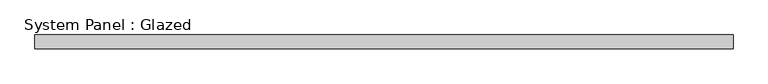
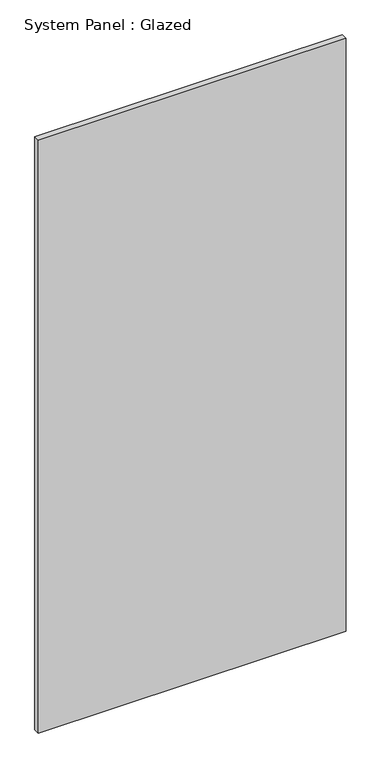
"""IFC4 building model written with IfcOpenShell, lengths in millimetres: plate geometry, System Panel : Glazed."""

from ifc_helpers import new_model, si_unit, origin, origin_with_axes, place, context, project, spatial, polyline, outline, extrude, source, transform, mapped, element, save


def system_panel_glazed_120799d7(model_context):
    return source(origin(), model_context, "Body", "SweptSolid", [
        extrude(outline(polyline([(650.875, 19.05), (-650.875, 19.05), (-650.875, 44.45), (650.875, 44.45), (650.875, 19.05)])), origin_with_axes(), (0.0, 0.0, 1.0), 2647.95),
    ])


if __name__ == "__main__":
    model = new_model("IFC4")
    model_context = context("Model", 3, world=origin())
    ifc_project = project(units=[si_unit("LENGTHUNIT", "METRE", prefix="MILLI")], contexts=[model_context])
    site = spatial("IfcSite", under=ifc_project)
    building = spatial("IfcBuilding", under=site)
    placement = place(None, origin())
    system_panel_glazed_shape = system_panel_glazed_120799d7(model_context)
    element("IfcPlate", 1, ObjectType="System Panel : Glazed", at=placement, inside=building, context=model_context, shape_type="MappedRepresentation", body=[
        mapped(system_panel_glazed_shape, transform((0.0, 0.0, 0.0), x_axis=(1.0, 0.0, 0.0), y_axis=(0.0, 1.0, 0.0), z_axis=(0.0, 0.0, 1.0))),
    ])
    save(model, "model.ifc")

# Revit data of these elements
# Type "System Panel : Glazed"
#   Construction Type Id = "GSP4R"
#   Analytic Construction = "1/8 in Pilkington single glazing"
#   Visual Light Transmittance = 0.9
#   Solar Heat Gain Coefficient = 0.86
#   Heat Transfer Coefficient (U) = 1.18115 BTU/(h·ft²·°F)
# Element 1 (IfcPlate, "System Panel : Glazed")
#   Materials on its faces: "Glass"
# Materials
#   "Glass": class "Glass", colour RGB 0 128 192, transparency 0.75, Description = "Soda Lime Glass", Cost = 0
